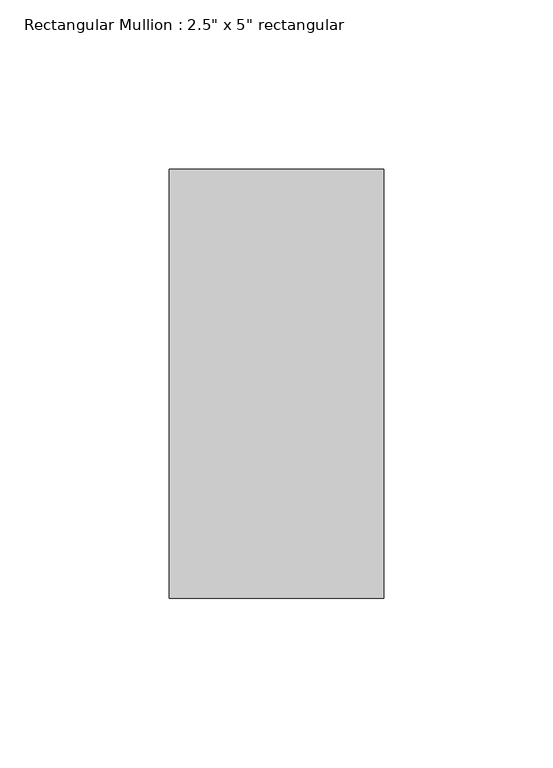
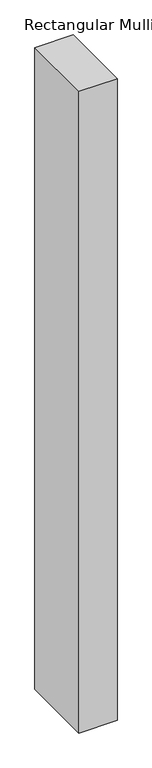
"""IFC4 building model written with IfcOpenShell, lengths in millimetres: member geometry."""

from ifc_helpers import new_model, si_unit, frame, origin, place, context, project, spatial, polyline, outline, extrude, source, transform, mapped, element, save


def member_c344cd1a(model_context):
    return source(origin(), model_context, "Body", "SweptSolid", [
        extrude(outline(polyline([(31.75, 63.5), (31.75, -63.5), (-31.75, -63.5), (-31.75, 63.5), (31.75, 63.5)])), frame((0.0, 0.0, -1130.2999998), z_axis=(0.0, 0.0, 1.0), x_axis=(1.0, 0.0, 0.0)), (0.0, 0.0, 1.0), 1130.2999998),
    ])


if __name__ == "__main__":
    model = new_model("IFC4")
    model_context = context("Model", 3, world=origin())
    ifc_project = project(units=[si_unit("LENGTHUNIT", "METRE", prefix="MILLI")], contexts=[model_context])
    site = spatial("IfcSite", under=ifc_project)
    building = spatial("IfcBuilding", under=site)
    placement = place(None, origin())
    member_shape = member_c344cd1a(model_context)
    element("IfcMember", 1, ObjectType="Rectangular Mullion : 2.5\" x 5\" rectangular", at=placement, inside=building, context=model_context, shape_type="MappedRepresentation", body=[
        mapped(member_shape, transform((0.0, 0.0, 0.0), x_axis=(1.0, 0.0, 0.0), y_axis=(0.0, 1.0, 0.0), z_axis=(0.0, 0.0, 1.0))),
    ])
    save(model, "model.ifc")

# Revit data of these elements
# Type "Rectangular Mullion : 2.5\" x 5\" rectangular"
#   built-in parameter 1007304 = 0.416667 (stored number, unit not read)
#   built-in parameter 1007301 = 0.104167 (stored number, unit not read)
#   built-in parameter 1007300 = 0.104167 (stored number, unit not read)
# Element 1 (IfcMember, "Rectangular Mullion : 2.5\" x 5\" rectangular")
#   Materials on its faces: "BLACK COLOUR"
# Materials
#   "BLACK COLOUR": class "Generic", colour RGB 120 120 120, transparency 0, Cost = 0
